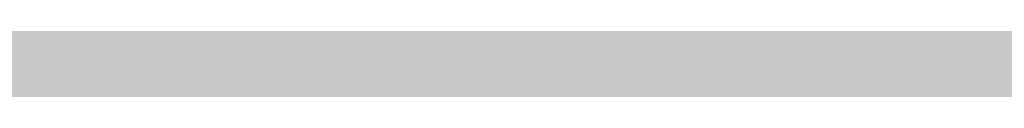
# Model space of a CAD drawing. Units: feet. Extents: x 3168 to 4724, y 827 to 1477.
# Tile 76 of 256: x 3273.3412 to 3273.6101, y 1099.0007 to 1099.0148. Entities that reach past the tile are written whole.
import ezdxf

# ---------------------------------------------------------------- set-up
doc = ezdxf.new("R2010")
doc.units = ezdxf.units.FT
doc.layers.add('A-ELEV', color=7, linetype='Continuous', lineweight=35)
doc.layers.add('A-ELEV-PATT', color=8, linetype='Continuous', lineweight=13)

msp = doc.modelspace()

# ---------------------------------------------------------------- hatches: boundary and pattern name
at = {"layer": 'A-ELEV-PATT'}
h = msp.add_hatch(color=256, dxfattribs=at)
h.dxf.hatch_style = 1
edge = h.paths.add_edge_path()
edge.add_ellipse((3552.90576, 979.22014), major_axis=(36.74492, 0), ratio=0.48484848, start_angle=0, end_angle=360)
edge = h.paths.add_edge_path()
edge.add_ellipse((3559.89164, 929.25228), major_axis=(36.74492, 0), ratio=0.48484848, start_angle=0, end_angle=360)
edge = h.paths.add_edge_path()
edge.add_line((3299.31681, 1198.60608), (3479.91671, 1198.60608))
edge.add_line((3479.91671, 1198.60608), (3479.91671, 1209.86857))
edge.add_spline(control_points=[(3479.91671, 1209.86857), (3464.30116, 1209.86857), (3448.6856, 1209.86857), (3410.94914, 1209.86857), (3388.82823, 1209.86857), (3355.64688, 1209.86857), (3344.58642, 1209.86857), (3327.99574, 1209.86857), (3322.46552, 1209.86857), (3314.17018, 1209.86857), (3311.40507, 1209.86857), (3307.2574, 1209.86857), (3305.87484, 1209.86857), (3303.801, 1209.86857), (3303.10973, 1209.86857), (3302.07281, 1209.86857), (3301.72717, 1209.86857), (3301.20871, 1209.86857), (3301.03589, 1209.86857), (3300.77666, 1209.86857), (3300.69025, 1209.86857), (3300.56064, 1209.86857), (3300.51743, 1209.86857), (3300.45263, 1209.86857), (3300.43102, 1209.86857), (3300.39862, 1209.86857), (3300.38782, 1209.86857), (3300.36622, 1209.86857), (3300.34568, 1209.86857), (3300.34555, 1209.86857), (3300.3455, 1209.86857), (3300.3433, 1209.86857), (3300.34115, 1209.86857), (3300.33791, 1209.86857), (3300.33683, 1209.86857), (3300.33394, 1209.86857), (3300.33213, 1209.86857), (3300.32552, 1209.86858), (3300.32071, 1209.86858), (3300.31092, 1209.86859), (3300.30595, 1209.8686), (3300.29051, 1209.86862), (3300.28005, 1209.86865), (3300.23243, 1209.86878), (3300.1953, 1209.86895), (3299.95107, 1209.87061), (3299.74482, 1209.87433), (3299.43683, 1209.88326), (3299.33439, 1209.88679), (3299.18108, 1209.89292), (3299.13003, 1209.8951), (3298.65222, 1209.9168), (3298.22946, 1209.94572), (3297.60163, 1210.00237), (3297.3934, 1210.02346), (3297.08265, 1210.05831), (3296.97933, 1210.07046), (3296.29295, 1210.15486), (3295.71815, 1210.24336), (3294.86872, 1210.39885), (3294.5877, 1210.45448), (3294.16934, 1210.54335), (3294.03042, 1210.57388), (3291.70715, 1211.1012), (3289.65359, 1211.81344), (3285.77626, 1213.56399), (3283.95141, 1214.60348), (3280.51216, 1216.98008), (3278.89724, 1218.31759), (3276.37991, 1220.82949), (3275.41604, 1221.91774), (3274.03934, 1223.7077), (3273.58104, 1224.34953), (3273.14323, 1225.01632)], knot_values=[39.119033, 39.119033, 39.119033, 39.119033, 39.286353, 39.286353, 39.523379, 39.523379, 39.641892, 39.641892, 39.701148, 39.701148, 39.730777, 39.730777, 39.745591, 39.745591, 39.752998, 39.752998, 39.756701, 39.756701, 39.758553, 39.758553, 39.759479, 39.759479, 39.759942, 39.759942, 39.760173, 39.760173, 39.760289, 39.760289, 39.760405, 39.760405, 39.760463, 39.760463, 39.763389, 39.763389, 39.764851, 39.764851, 39.767304, 39.767304, 39.773825, 39.773825, 39.78057, 39.78057, 39.79477, 39.79477, 39.845194, 39.845194, 40.126715, 40.126715, 40.267476, 40.267476, 40.337856, 40.337856, 40.927023, 40.927023, 41.221606, 41.221606, 41.368898, 41.368898, 42.202622, 42.202622, 42.619485, 42.619485, 42.827916, 42.827916, 46.118323, 46.118323, 49.408731, 49.408731, 52.699139, 52.699139, 54.927489, 54.927489, 56.104228, 56.104228, 56.104228, 56.104228], weights=[1, 1, 1, 1, 1, 1, 1, 1, 1, 1, 1, 1, 1, 1, 1, 1, 1, 1, 1, 1, 1, 1, 1, 1, 1, 1, 1, 1, 1, 1, 1, 1, 1, 1, 1, 1, 1, 1, 1, 1, 1, 1, 1, 1, 1, 1, 1, 1, 1, 1, 1, 1, 1, 1, 1, 1, 1, 1, 1, 1, 1, 1, 1, 1, 1, 1, 1, 1, 1, 1, 1, 1, 1, 1], degree=3, periodic=0)
edge.add_line((3273.14323, 1225.01632), (3273.14323, 1099.01632))
edge.add_line((3273.14323, 1099.01632), (3299.31681, 1099.01632))
edge.add_line((3299.31681, 1099.01632), (3299.31681, 1198.60608))
edge = h.paths.add_edge_path()
edge.add_line((3304.75844, 1324.15806), (3479.91671, 1324.15806))
edge.add_line((3479.91671, 1324.15806), (3479.91671, 1335.71462))
edge.add_line((3479.91671, 1335.71462), (3269.16163, 1335.71462))
edge.add_spline(control_points=[(3269.16163, 1335.71462), (3264.02423, 1335.71462), (3258.36412, 1328.95819), (3259.26431, 1323.90027)], knot_values=[0, 0, 0, 0, 15.412191, 15.412191, 15.412191, 15.412191], degree=3, periodic=0)
edge.add_line((3259.26431, 1323.90027), (3265.51685, 1288.76913))
edge.add_line((3265.51685, 1288.76913), (3275.2651, 1261.54563))
edge.add_line((3275.2651, 1261.54563), (3304.75844, 1261.54563))
edge.add_line((3304.75844, 1261.54563), (3304.75844, 1324.15806))
h = msp.add_hatch(color=256, dxfattribs=at)
h.dxf.hatch_style = 1
h.paths.add_polyline_path([(3384.52525, 1099.01632), (3335.02917, 1099.01632), (3299.31681, 1099.01632), (3273.14323, 1099.01632), (3217.56536, 1099.01632), (3168.06928, 827.11626), (3335.02917, 827.11626)])

# ---------------------------------------------------------------- linework, layer by layer
at = {"layer": 'A-ELEV'}
msp.add_open_spline([(3808.5202, 1099.01632), (3808.5202, 1141.41324), (3808.5202, 1183.81015), (3808.5202, 1226.63532), (3808.5202, 1227.06358), (3808.5202, 1227.49183), (3811.49187, 1248.99467), (3814.46354, 1270.49752), (3817.46523, 1292.21756), (3817.49525, 1292.43476), (3817.52526, 1292.65196), (3817.5728, 1310.10675), (3817.62034, 1327.56153), (3817.66788, 1345.01632), (3817.66788, 1345.45796), (3817.66788, 1345.89961), (3817.66788, 1346.45605), (3817.66788, 1346.57084), (3817.66788, 1346.75289), (3817.66788, 1346.82014), (3817.66788, 1346.93487), (3817.66788, 1346.98234), (3817.66788, 1347.03859), (3817.66788, 1347.04736), (3817.66788, 1347.07366), (3817.66788, 1347.0593), (3817.66788, 1347.06155), (3817.66788, 1347.06267), (3817.66788, 1347.06603), (3817.66787, 1347.06827), (3817.66787, 1347.075), (3817.66787, 1347.07949), (3817.66785, 1347.09294), (3817.66783, 1347.1019), (3817.66777, 1347.12879), (3817.6677, 1347.1467), (3817.66743, 1347.20042), (3817.66716, 1347.23619), (3817.6661, 1347.34338), (3817.66504, 1347.41469), (3817.66081, 1347.62809), (3817.65661, 1347.76971), (3817.63997, 1348.19249), (3817.62351, 1348.47159), (3817.55909, 1349.30007), (3817.49612, 1349.84059), (3817.25543, 1351.42416), (3817.02632, 1352.42879), (3816.30687, 1354.88891), (3815.74375, 1356.26873), (3814.46396, 1358.81921), (3813.74641, 1359.99097), (3812.19584, 1362.17234), (3811.36225, 1363.18212), (3809.58884, 1365.06901), (3808.64882, 1365.94611), (3806.65426, 1367.57962), (3805.5997, 1368.33615), (3803.35289, 1369.72233), (3802.16054, 1370.35239), (3799.60081, 1371.45359), (3798.23269, 1371.92548), (3795.28008, 1372.63462), (3793.69315, 1372.87207), (3791.86944, 1372.92648), (3791.74086, 1372.92922), (3791.35337, 1372.9341), (3791.09271, 1372.9329), (3790.30412, 1372.91507), (3789.76954, 1372.88419), (3789.20919, 1372.83024), (3789.19062, 1372.82842), (3789.13489, 1372.82291), (3789.0977, 1372.81914), (3789.04844, 1372.81401), (3789.0364, 1372.81274), (3789.00026, 1372.80892), (3788.97615, 1372.80633), (3788.9494, 1372.8034), (3788.94679, 1372.80312), (3788.94257, 1372.80266), (3788.94097, 1372.80248), (3788.93857, 1372.80222), (3788.93778, 1372.80213), (3788.93539, 1372.80187), (3788.86753, 1372.7944), (3788.75687, 1372.78223), (3788.70153, 1372.77614), (3788.53553, 1372.75788), (3788.42486, 1372.74571), (3788.09286, 1372.70918), (3787.87152, 1372.68484), (3787.20751, 1372.61179), (3786.76483, 1372.5631), (3785.43681, 1372.41701), (3784.55147, 1372.31962), (3781.89542, 1372.02744), (3780.12473, 1371.83266), (3774.81265, 1371.24831), (3771.27126, 1370.85874), (3760.64709, 1369.69004), (3753.56431, 1368.9109), (3732.31597, 1366.5735), (3718.15042, 1365.01523), (3694.00676, 1362.35933), (3684.02866, 1361.26169), (3674.05056, 1360.16406), (3664.60066, 1360.16406), (3655.15077, 1360.16406), (3626.80108, 1360.16406), (3607.90129, 1360.16406), (3551.20192, 1360.16406), (3513.40234, 1360.16406), (3467.72518, 1360.16406), (3459.8476, 1360.16406), (3436.21487, 1360.16406), (3420.45972, 1360.16406), (3373.19425, 1360.16406), (3341.68395, 1360.16406), (3302.84816, 1360.16406), (3295.52269, 1360.16406), (3286.03829, 1360.16406), (3283.87937, 1360.16406), (3277.40261, 1360.16406), (3273.08477, 1360.16406), (3267.73285, 1360.16406), (3266.69877, 1360.16406), (3263.59652, 1360.16406), (3261.52835, 1360.16406), (3259.23694, 1360.16406), (3259.0137, 1360.16406), (3258.34396, 1360.16406), (3257.89747, 1360.16406), (3257.431, 1360.16406), (3257.41102, 1360.16406), (3257.37057, 1360.16406), (3257.37547, 1360.16406), (3257.3746, 1360.16406), (3257.37394, 1360.16406), (3257.37196, 1360.16406), (3257.37064, 1360.16406), (3257.36667, 1360.16406), (3257.36403, 1360.16406), (3257.35611, 1360.16405), (3257.35083, 1360.16405), (3257.33499, 1360.16402), (3257.32443, 1360.164), (3257.29277, 1360.1639), (3257.27168, 1360.1638), (3257.20844, 1360.1634), (3257.16634, 1360.163), (3257.04021, 1360.16139), (3256.95635, 1360.15978), (3256.7055, 1360.15339), (3256.53924, 1360.14704), (3256.04357, 1360.12192), (3255.7173, 1360.0971), (3254.75245, 1360.00048), (3254.12797, 1359.90651), (3252.18007, 1359.52533), (3250.94157, 1359.14399), (3248.67018, 1358.24329), (3247.63574, 1357.72383), (3245.73263, 1356.60347), (3244.86339, 1356.00206), (3243.25311, 1354.74287), (3242.51197, 1354.08473), (3240.75105, 1352.34478), (3239.80096, 1351.22957), (3238.08777, 1348.87244), (3237.32469, 1347.63036), (3235.98251, 1344.97163), (3235.40221, 1343.55491), (3234.59108, 1340.81546), (3234.31088, 1339.54355), (3233.97649, 1336.80256), (3233.92211, 1335.33088), (3234.14892, 1332.59127), (3234.34953, 1331.3672), (3234.71989, 1329.99937), (3234.75242, 1329.88336), (3234.85362, 1329.5348), (3234.92589, 1329.30168), (3235.02484, 1329.00255), (3235.04692, 1328.93693), (3235.07764, 1328.84724), (3235.08592, 1328.8232), (3235.11094, 1328.75106), (3235.12783, 1328.70296), (3235.14799, 1328.64624), (3235.15106, 1328.63763), (3235.1561, 1328.62353), (3235.15806, 1328.61803), (3235.16021, 1328.61203), (3235.16561, 1328.59694), (3235.1801, 1328.55649), (3235.19026, 1328.5281), (3235.22076, 1328.44295), (3235.24108, 1328.38618), (3235.30207, 1328.21587), (3235.34273, 1328.10232), (3235.4647, 1327.7617), (3235.54601, 1327.53462), (3235.78995, 1326.85338), (3235.95258, 1326.39922), (3236.44046, 1325.03674), (3236.76571, 1324.12841), (3237.74148, 1321.40345), (3238.39198, 1319.5868), (3240.34351, 1314.13687), (3241.64452, 1310.50358), (3245.54757, 1299.60371), (3248.14961, 1292.33713), (3255.95571, 1270.53739), (3261.15977, 1256.00423), (3267.38762, 1238.612), (3268.4114, 1235.75294), (3269.51038, 1232.68386), (3269.58558, 1232.47385), (3269.70661, 1232.13585), (3269.75244, 1232.00786), (3269.82733, 1231.79873), (3269.85638, 1231.7176), (3269.90632, 1231.57812), (3269.92721, 1231.51978), (3269.97247, 1231.39341), (3269.99683, 1231.32537), (3270.0265, 1231.24251), (3270.03181, 1231.22768), (3270.04028, 1231.20402), (3270.03922, 1231.20698), (3270.03936, 1231.2066), (3270.03943, 1231.20641), (3270.03963, 1231.20585), (3270.03977, 1231.20547), (3270.04017, 1231.20433), (3270.04044, 1231.20358), (3270.04125, 1231.20131), (3270.0418, 1231.1998), (3270.04342, 1231.19527), (3270.0445, 1231.19225), (3270.04776, 1231.18318), (3270.04993, 1231.17714), (3270.05644, 1231.15903), (3270.06079, 1231.14696), (3270.07387, 1231.11076), (3270.08261, 1231.08666), (3270.10894, 1231.01441), (3270.1266, 1230.96635), (3270.17993, 1230.82246), (3270.21595, 1230.72692), (3270.32532, 1230.44151), (3270.40003, 1230.25281), (3270.62925, 1229.69144), (3270.78888, 1229.3235), (3271.28649, 1228.23832), (3271.6431, 1227.53975), (3272.77586, 1225.51528), (3273.61417, 1224.2605), (3275.41604, 1221.91774), (3276.37991, 1220.82949), (3278.89724, 1218.31759), (3280.51216, 1216.98008), (3283.95141, 1214.60348), (3285.77626, 1213.56399), (3289.65359, 1211.81344), (3291.70715, 1211.1012), (3294.03042, 1210.57388), (3294.16934, 1210.54335), (3294.5877, 1210.45448), (3294.86872, 1210.39885), (3295.71815, 1210.24336), (3296.29295, 1210.15486), (3296.97933, 1210.07046), (3297.08265, 1210.05831), (3297.3934, 1210.02346), (3297.60163, 1210.00237), (3298.22946, 1209.94572), (3298.65222, 1209.9168), (3299.13003, 1209.8951), (3299.18108, 1209.89292), (3299.33439, 1209.88679), (3299.43683, 1209.88326), (3299.74482, 1209.87433), (3299.95107, 1209.87061), (3300.1953, 1209.86895), (3300.23243, 1209.86878), (3300.28005, 1209.86865), (3300.29051, 1209.86862), (3300.30595, 1209.8686), (3300.31092, 1209.86859), (3300.32071, 1209.86858), (3300.32552, 1209.86858), (3300.33213, 1209.86857), (3300.33394, 1209.86857), (3300.33683, 1209.86857), (3300.33791, 1209.86857), (3300.34115, 1209.86857), (3300.3433, 1209.86857), (3300.3455, 1209.86857), (3300.34555, 1209.86857), (3300.34568, 1209.86857), (3300.36622, 1209.86857), (3300.38782, 1209.86857), (3300.39862, 1209.86857), (3300.43102, 1209.86857), (3300.45263, 1209.86857), (3300.51743, 1209.86857), (3300.56064, 1209.86857), (3300.69025, 1209.86857), (3300.77666, 1209.86857), (3301.03589, 1209.86857), (3301.20871, 1209.86857), (3301.72717, 1209.86857), (3302.07281, 1209.86857), (3303.10973, 1209.86857), (3303.801, 1209.86857), (3305.87484, 1209.86857), (3307.2574, 1209.86857), (3311.40507, 1209.86857), (3314.17018, 1209.86857), (3322.46552, 1209.86857), (3327.99574, 1209.86857), (3344.58642, 1209.86857), (3355.64688, 1209.86857), (3388.82823, 1209.86857), (3410.94914, 1209.86857), (3477.31185, 1209.86857), (3521.55366, 1209.86857), (3566.83618, 1209.86857), (3567.87689, 1209.86857), (3570.99902, 1209.86857), (3573.08043, 1209.86857), (3575.7814, 1209.86857), (3576.40094, 1209.86857), (3577.29582, 1209.86857), (3577.57115, 1209.86857), (3578.39715, 1209.86857), (3578.94781, 1209.86857), (3579.75649, 1209.86857), (3580.01451, 1209.86857), (3580.34274, 1209.86857), (3580.32686, 1209.86857), (3580.32717, 1209.86857), (3580.32732, 1209.86857), (3580.32778, 1209.86857), (3580.32809, 1209.86857), (3580.329, 1209.86857), (3580.32961, 1209.86857), (3580.33145, 1209.86857), (3580.33267, 1209.86857), (3580.33633, 1209.86857), (3580.33878, 1209.86857), (3580.34611, 1209.86856), (3580.35099, 1209.86856), (3580.36566, 1209.86854), (3580.37544, 1209.86852), (3580.4048, 1209.86845), (3580.42439, 1209.86838), (3580.48318, 1209.86808), (3580.52244, 1209.86779), (3580.64036, 1209.86662), (3580.71919, 1209.86545), (3580.95632, 1209.86077), (3581.11522, 1209.85607), (3581.59416, 1209.83723), (3581.91642, 1209.81833), (3582.88995, 1209.74243), (3583.54799, 1209.66617), (3585.53183, 1209.36062), (3586.86722, 1209.05389), (3589.47155, 1208.25247), (3590.74024, 1207.75785), (3591.99545, 1207.1588), (3592.05781, 1207.12874), (3592.24424, 1207.03795), (3592.36768, 1206.97663), (3592.73528, 1206.79036), (3592.97675, 1206.6631), (3593.24454, 1206.51644), (3593.27473, 1206.49982), (3593.36512, 1206.44984), (3593.42511, 1206.41633), (3593.60431, 1206.31529), (3593.72273, 1206.24721), (3593.85721, 1206.1684), (3593.87436, 1206.15832), (3593.92574, 1206.12804), (3593.9599, 1206.1078), (3594.06209, 1206.0469), (3594.12983, 1206.00607), (3594.20844, 1205.95817), (3594.21968, 1205.9513), (3594.25339, 1205.93069), (3594.27582, 1205.91692), (3594.34297, 1205.87554), (3594.38756, 1205.84785), (3594.43362, 1205.81905), (3594.43526, 1205.81802), (3594.44017, 1205.81495), (3594.44345, 1205.81289), (3594.44712, 1205.81059), (3594.44752, 1205.81035), (3594.44869, 1205.80961), (3594.44948, 1205.80912), (3594.45037, 1205.80856), (3594.45047, 1205.8085), (3594.4506, 1205.80842), (3594.4674, 1205.79789), (3594.49327, 1205.78167), (3594.5062, 1205.77357), (3594.54501, 1205.74925), (3594.57088, 1205.73303), (3594.64849, 1205.6844), (3594.70023, 1205.65197), (3594.85544, 1205.55469), (3594.95892, 1205.48984), (3595.26936, 1205.29528), (3595.47631, 1205.16558), (3596.09719, 1204.77646), (3596.5111, 1204.51705), (3597.75284, 1203.73883), (3598.58067, 1203.22001), (3601.06415, 1201.66355), (3602.71981, 1200.62591), (3607.68677, 1197.513), (3610.99809, 1195.43773), (3620.93202, 1189.2119), (3627.55464, 1185.06135), (3647.42251, 1172.60971), (3660.66775, 1164.30861), (3700.40348, 1139.40531), (3726.89397, 1122.80312), (3757.20572, 1103.80605), (3761.02697, 1101.41118), (3764.84822, 1099.01632), (3745.32827, 1099.01632), (3725.80832, 1099.01632), (3706.28837, 1099.01632), (3706.28837, 1108.45324), (3706.28837, 1117.89016), (3706.28837, 1127.32708), (3710.75075, 1127.32708), (3715.21314, 1127.32708), (3719.67553, 1127.32708)], degree=3, knots=[0, 0, 0, 0, 0.982037, 0.982037, 0.991957, 0.991957, 0.991957, 1.966522, 1.966522, 1.976367, 1.976367, 1.976367, 2.976367, 2.976367, 2.976367, 3.00169, 3.00169, 3.008272, 3.008272, 3.012129, 3.012129, 3.014851, 3.014851, 3.015353, 3.015353, 3.016359, 3.016359, 3.017365, 3.017365, 3.019376, 3.019376, 3.023398, 3.023398, 3.031442, 3.031442, 3.047531, 3.047531, 3.079708, 3.079708, 3.144063, 3.144063, 3.272772, 3.272772, 3.53019, 3.53019, 4.045026, 4.045026, 5.074698, 5.074698, 6.700878, 6.700878, 8.327058, 8.327058, 9.953238, 9.953238, 11.579418, 11.579418, 13.205598, 13.205598, 14.831778, 14.831778, 16.457958, 16.457958, 18.084138, 18.084138, 18.206872, 18.206872, 18.45234, 18.45234, 18.943275, 18.943275, 18.960093, 18.960093, 18.993729, 18.993729, 19.00461, 19.00461, 19.026374, 19.026374, 19.028737, 19.028737, 19.03018, 19.03018, 19.030897, 19.030897, 19.032332, 19.032332, 19.033766, 19.033766, 19.036636, 19.036636, 19.042374, 19.042374, 19.053851, 19.053851, 19.076805, 19.076805, 19.122714, 19.122714, 19.21453, 19.21453, 19.398163, 19.398163, 19.765429, 19.765429, 20.024128, 20.024128, 20.024128, 20.092031, 20.092031, 20.227836, 20.227836, 20.499446, 20.499446, 20.556051, 20.556051, 20.66926, 20.66926, 20.895678, 20.895678, 20.948316, 20.948316, 20.963829, 20.963829, 20.994855, 20.994855, 21.002285, 21.002285, 21.017146, 21.017146, 21.01875, 21.01875, 21.021959, 21.021959, 21.022102, 21.022102, 21.022249, 21.022249, 21.022708, 21.022708, 21.023627, 21.023627, 21.025464, 21.025464, 21.029138, 21.029138, 21.036486, 21.036486, 21.051183, 21.051183, 21.080575, 21.080575, 21.139361, 21.139361, 21.256932, 21.256932, 21.492073, 21.492073, 21.962356, 21.962356, 23.01002, 23.01002, 24.057684, 24.057684, 25.105348, 25.105348, 26.153011, 26.153011, 27.776787, 27.776787, 29.400562, 29.400562, 31.024337, 31.024337, 32.278801, 32.278801, 33.533265, 33.533265, 34.467568, 34.467568, 34.553971, 34.553971, 34.726776, 34.726776, 34.775309, 34.775309, 34.793079, 34.793079, 34.82862, 34.82862, 34.834979, 34.834979, 34.839039, 34.839039, 34.839411, 34.839411, 34.840285, 34.840285, 34.842034, 34.842034, 34.845531, 34.845531, 34.852525, 34.852525, 34.866512, 34.866512, 34.894488, 34.894488, 34.950439, 34.950439, 35.062342, 35.062342, 35.286147, 35.286147, 35.733758, 35.733758, 35.821815, 35.821815, 35.828283, 35.828283, 35.832225, 35.832225, 35.834724, 35.834724, 35.836521, 35.836521, 35.838617, 35.838617, 35.839073, 35.839073, 35.839345, 35.839345, 35.839617, 35.839617, 35.840161, 35.840161, 35.841249, 35.841249, 35.843425, 35.843425, 35.847778, 35.847778, 35.856482, 35.856482, 35.873891, 35.873891, 35.908709, 35.908709, 35.978345, 35.978345, 36.117617, 36.117617, 36.396161, 36.396161, 36.953248, 36.953248, 38.067423, 38.067423, 40.295772, 40.295772, 42.524122, 42.524122, 45.81453, 45.81453, 49.104937, 49.104937, 52.395345, 52.395345, 52.603776, 52.603776, 53.020639, 53.020639, 53.854363, 53.854363, 54.001655, 54.001655, 54.296238, 54.296238, 54.885405, 54.885405, 54.955785, 54.955785, 55.096546, 55.096546, 55.378067, 55.378067, 55.42849, 55.42849, 55.442691, 55.442691, 55.449436, 55.449436, 55.455957, 55.455957, 55.458409, 55.458409, 55.459872, 55.459872, 55.462798, 55.462798, 55.462856, 55.462856, 55.462972, 55.462972, 55.463088, 55.463088, 55.463319, 55.463319, 55.463782, 55.463782, 55.464708, 55.464708, 55.46656, 55.46656, 55.470263, 55.470263, 55.47767, 55.47767, 55.492484, 55.492484, 55.522112, 55.522112, 55.581369, 55.581369, 55.699882, 55.699882, 55.936907, 55.936907, 56.410959, 56.410959, 56.42211, 56.42211, 56.444413, 56.444413, 56.451051, 56.451051, 56.454001, 56.454001, 56.459901, 56.459901, 56.462666, 56.462666, 56.463418, 56.463418, 56.464171, 56.464171, 56.465675, 56.465675, 56.468684, 56.468684, 56.474702, 56.474702, 56.486738, 56.486738, 56.51081, 56.51081, 56.558955, 56.558955, 56.655243, 56.655243, 56.847821, 56.847821, 57.232975, 57.232975, 58.003284, 58.003284, 59.543901, 59.543901, 62.625137, 62.625137, 68.787607, 68.787607, 74.950078, 74.950078, 75.27336, 75.27336, 75.919923, 75.919923, 77.213051, 77.213051, 77.377769, 77.377769, 77.707206, 77.707206, 78.366079, 78.366079, 78.462532, 78.462532, 78.655436, 78.655436, 79.041245, 79.041245, 79.105735, 79.105735, 79.234714, 79.234714, 79.492672, 79.492672, 79.502197, 79.502197, 79.521249, 79.521249, 79.523534, 79.523534, 79.528103, 79.528103, 79.528682, 79.528682, 79.528885, 79.528885, 79.529089, 79.529089, 79.529495, 79.529495, 79.530308, 79.530308, 79.531935, 79.531935, 79.535187, 79.535187, 79.541693, 79.541693, 79.554704, 79.554704, 79.580725, 79.580725, 79.632769, 79.632769, 79.736856, 79.736856, 79.94503, 79.94503, 80.361377, 80.361377, 80.421435, 80.421435, 80.421435, 81.421435, 81.421435, 81.421435, 82.421435, 82.421435, 82.421435, 83.421435, 83.421435, 83.421435, 83.421435], dxfattribs=at)

doc.saveas('drawing.dxf')
